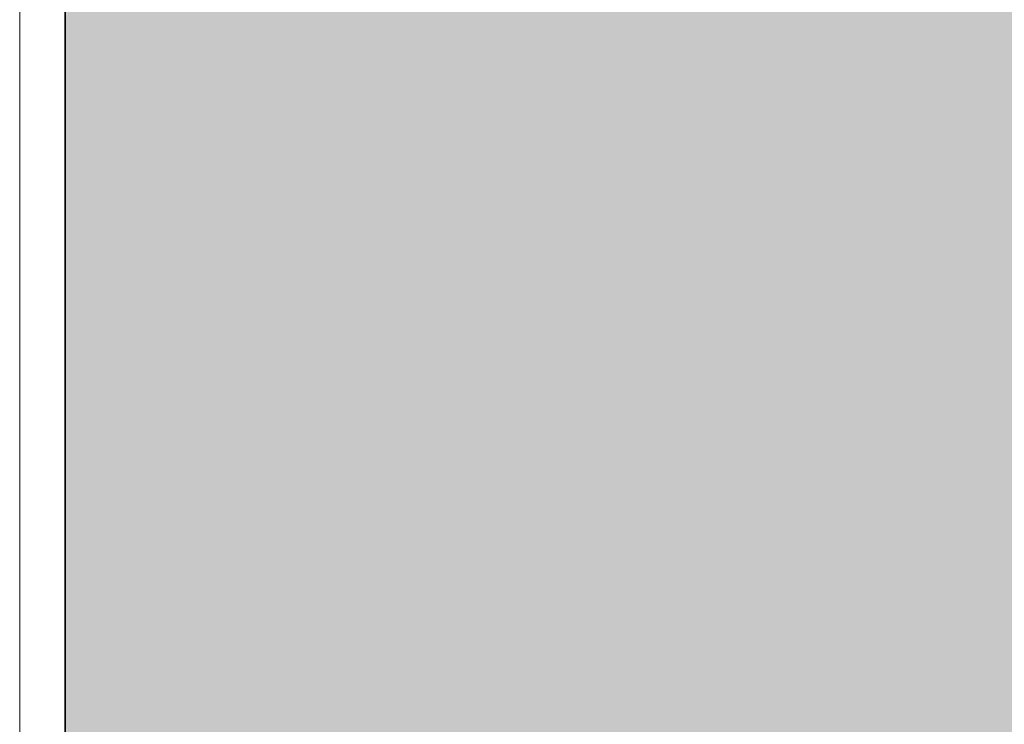
# Model space of a CAD drawing. Units: inches. Extents: x 2091 to 2899, y 967 to 2217.
# Tile 234 of 256: x 2203.1157 to 2203.7172, y 1152.6774 to 1153.1078. Entities that reach past the tile are written whole.
import ezdxf

# ---------------------------------------------------------------- set-up
doc = ezdxf.new("R2010")
doc.units = ezdxf.units.IN
doc.layers.add('A-GLAZ', color=4, linetype='Continuous', lineweight=18)
doc.layers.add('C-PROP', color=7, linetype='Continuous', lineweight=35)
doc.layers.add('A-WALL-PATT', color=141, linetype='Continuous', lineweight=13, true_color=0xadddf7)

# ---------------------------------------------------------------- blocks, each defined once
blk = doc.blocks.new('WIN-DOUBLE-LINE')
blk.add_line((0.0004, -0.00045), (0.0004, 80.8229))

msp = doc.modelspace()

# ---------------------------------------------------------------- hatches: boundary and pattern name
at = {"layer": 'A-WALL-PATT'}
h = msp.add_hatch(color=256, dxfattribs=at)
h.dxf.hatch_style = 1
h.paths.add_polyline_path([(2803.1436, 2050.91906), (2203.1436, 2050.91906), (2203.1436, 1090.91906), (2803.1436, 1090.91906)])
h.paths.add_polyline_path([(2635.79885, 1147.54046), (2674.52405, 1147.54046, 0.376086), (2678.52967, 1152.8802), (2678.52967, 1159.55647, 0.333335), (2674.52432, 1163.56185), (2674.52432, 1163.56185), (2674.52432, 1192.93439), (2635.80597, 1192.93439), (2597.08762, 1192.93439), (2597.08762, 1163.56185, 0.333335), (2593.08228, 1159.55647), (2593.08228, 1152.8802, 0.376086), (2597.08789, 1147.54046)], flags=0)
h.paths.add_polyline_path([(2436.01043, 1278.24078, 0.000483), (2435.95264, 1278.21503, -0.001328), (2435.93563, 1278.11169, -0.001711), (2436.11644, 1278.04076, 0.002185)], flags=0)
h.paths.add_polyline_path([(2794.1436, 1143.41906), (2794.1436, 1347.41906), (2543.37017, 1347.41906), (2543.37017, 1351.91906), (2794.1436, 1351.91906), (2794.1436, 1392.71355), (2793.9474, 1392.71355), (2793.9474, 1473.5369), (2794.1436, 1473.5369), (2794.1436, 1531.91906), (2650.1436, 1531.91906), (2650.1436, 1536.41906), (2794.1436, 1536.41906), (2794.1436, 1692.41906), (2609.37561, 1692.41906), (2609.37561, 1644.41906), (2604.87561, 1644.41906), (2604.87561, 1744.91906), (2609.37561, 1744.91906), (2609.37561, 1696.91906), (2794.1436, 1696.91906), (2794.1436, 1780.91906), (2609.6436, 1780.91906), (2493.87561, 1780.91906), (2493.87561, 1785.41906), (2609.6436, 1785.41906), (2794.1436, 1785.41906), (2794.1436, 1847.93882), (2793.95122, 1847.93882), (2793.95122, 1928.76217), (2794.1436, 1928.76217), (2794.1436, 1941.41906), (2614.1436, 1941.41906), (2614.1436, 1821.41906), (2609.6436, 1821.41906), (2609.6436, 1941.41906), (2392.1436, 1941.41906), (2392.1436, 1819.91906), (2387.6436, 1819.91906), (2387.6436, 1941.41906), (2212.1436, 1941.41906), (2212.1436, 1783.91906), (2392.1436, 1783.91906), (2392.1436, 1780.91906), (2212.1436, 1780.91906), (2212.1436, 1629.41906), (2387.6436, 1629.41906), (2387.6436, 1744.91906), (2392.1436, 1744.91906), (2392.1436, 1627.91906), (2317.1436, 1627.91906), (2317.1436, 1551.41906), (2317.1436, 1536.41906), (2459.38359, 1536.41906), (2459.38359, 1602.39648), (2463.88359, 1602.39648), (2463.88359, 1531.91906), (2456.6436, 1531.91906), (2456.6436, 1529.91906), (2452.1436, 1529.91906), (2452.1436, 1531.91906), (2312.6436, 1531.91906), (2312.6436, 1551.41906), (2306.1436, 1551.41906), (2306.1436, 1555.91906), (2308.1436, 1555.91906), (2308.1436, 1551.41906), (2312.6436, 1551.41906), (2312.6436, 1627.91906), (2212.1436, 1627.91906), (2212.1436, 1555.91906), (2270.1436, 1555.91906), (2270.1436, 1551.41906), (2212.1436, 1551.41906), (2212.1436, 1351.91906), (2272.1436, 1351.91906), (2272.1436, 1347.41906), (2212.1436, 1347.41906), (2212.1436, 1275.41906), (2308.1436, 1275.41906), (2308.1436, 1351.91906), (2452.1436, 1351.91906), (2452.1436, 1493.91906), (2456.6436, 1493.91906), (2456.6436, 1347.41906), (2312.6436, 1347.41906), (2312.6436, 1270.91906), (2212.1436, 1270.91906), (2212.1436, 1099.91906), (2281.23752, 1099.91906), (2282.87104, 1110.9138), (2282.00834, 1116.9966), (2278.55774, 1121.4204), (2268.20564, 1128.0562), (2272.08764, 1128.0562), (2273.81294, 1131.927), (2279.42034, 1134.6919), (2285.02784, 1135.2449), (2287.61584, 1137.4568), (2288.04714, 1138.0098), (2289.34114, 1140.7747), (2291.06654, 1139.6687), (2292.36054, 1135.2449), (2295.37984, 1136.9038), (2296.24254, 1135.7979), (2297.10524, 1133.033), (2300.12464, 1138.0098), (2303.14394, 1138.0098), (2304.43794, 1135.7979), (2303.14394, 1133.586), (2306.59464, 1134.6919), (2307.88874, 1133.033), (2310.90804, 1135.2449), (2313.92744, 1134.1389), (2315.62686, 1132.4271), (2308.32004, 1117.5496), (2290.20384, 1109.8079), (2288.90984, 1103.1721), (2289.27231, 1099.91906), (2434.91823, 1099.91906), (2431.59323, 1124.78806), (2429.93023, 1169.55306), (2430.92718, 1240.51969), (2435.65893, 1238.18613), (2437.13523, 1196.55406), (2438.79823, 1143.97306), (2442.67823, 1111.99806), (2446.55823, 1099.91906), (2794.1436, 1099.91906), (2794.1436, 1138.91906), (2548.03245, 1138.91906), (2548.03245, 1143.41906), (2548.03245, 1148.81906), (2546.66846, 1148.03156), (2528.68569, 1179.17862, 0.256256), (2512.03245, 1148.81906), (2512.03245, 1143.41906), (2512.03245, 1138.91906), (2507.53245, 1138.91906), (2507.53245, 1143.41906), (2507.53245, 1148.81906, 0.256256), (2490.8792, 1179.17862), (2472.89644, 1148.03156), (2471.53245, 1148.81906), (2471.53245, 1143.41906), (2467.03245, 1143.41906), (2467.03245, 1269.94579, 0.039061), (2460.90999, 1273.58006), (2467.03245, 1273.58006), (2467.03245, 1286.32536, 0.014511), (2465.21619, 1286.76191), (2467.03245, 1287.05258), (2467.03245, 1323.41906), (2471.53245, 1323.41906), (2471.53245, 1148.81906), (2489.53245, 1179.99597), (2490.89644, 1179.20847), (2490.8792, 1179.17862, -0.256256), (2507.53245, 1148.81906), (2507.53245, 1143.41906), (2512.03245, 1143.41906), (2512.03245, 1148.81906, -0.256256), (2528.68569, 1179.17862), (2528.66846, 1179.20847), (2530.03245, 1179.99597), (2548.03245, 1148.81906), (2548.03245, 1143.41906)], flags=16)
h.paths.add_polyline_path([(2607.76855, 1200.94508), (2607.76855, 1265.03063), (2597.08762, 1281.05201), (2619.78459, 1281.05201), (2627.79528, 1337.12686), (2635.79885, 1337.12686), (2643.81666, 1337.12686), (2651.82736, 1281.05201), (2674.52432, 1281.05201), (2663.8434, 1265.03063), (2663.8434, 1200.94508), (2635.80597, 1200.94508)], flags=0)
edge = h.paths.add_edge_path(flags=0)
edge.add_ellipse((13303.89622, 1272.99872), major_axis=(-10595.31304, 0), ratio=0.84230387009, start_angle=0.628237219, end_angle=0.6465541, ccw=False)
edge.add_ellipse((2711.70045, 1156.85268), major_axis=(2.21977, 0), ratio=0.8423039, start_angle=111.53524, end_angle=180.62824, ccw=False)
edge.add_ellipse((13303.15629, 1272.99872), major_axis=(-10593.02631, 0), ratio=0.84230386954, start_angle=0.528271472, end_angle=0.646554097, ccw=False)
edge.add_line((2710.7646, 1175.3333), (2710.12999, 1175.3333))
edge.add_ellipse((2710.12999, 1176.57978), major_axis=(1.47985, 0), ratio=0.8423039, start_angle=180, end_angle=270, ccw=False)
edge.add_line((2708.65014, 1176.57978), (2708.65014, 1200.78291))
edge.add_ellipse((2710.12999, 1200.78291), major_axis=(1.47985, 0), ratio=0.8423039, start_angle=90, end_angle=180, ccw=False)
edge.add_line((2710.12999, 1202.02939), (2710.46508, 1202.02939))
edge.add_ellipse((13303.15629, 1272.99872), major_axis=(-10593.02631, 0), ratio=0.84230386954, start_angle=-0.090229089, end_angle=0.383866779, ccw=False)
edge.add_ellipse((2710.12999, 1290.92703), major_axis=(-1.47985, 0), ratio=0.8423039, start_angle=0, end_angle=90, ccw=False)
edge.add_line((2708.65014, 1290.92703), (2708.65014, 1315.13017))
edge.add_ellipse((2710.12999, 1315.13017), major_axis=(-1.47985, 0), ratio=0.8423039, start_angle=-90, end_angle=0, ccw=False)
edge.add_line((2710.12999, 1316.37665), (2710.70631, 1316.37665))
edge.add_ellipse((3238.40172, 1296.28957), major_axis=(528.234, 0), ratio=0.84230387, start_angle=176.3495724, end_angle=177.8200497, ccw=False)
edge.add_ellipse((2775.06304, 1071.4507), major_axis=(313.30776, 0), ratio=0.84230387, start_angle=102.1259656, end_angle=103.780529, ccw=False)
edge.add_ellipse((2775.06304, 1078.3057), major_axis=(-305.30289, 0), ratio=0.84230387, start_angle=-79.790461, end_angle=-77.5553727, ccw=False)
edge.add_ellipse((2695.14177, 1541.97538), major_axis=(-250.96022, 0), ratio=0.84230387, start_angle=99.256566, end_angle=102.5549326)
edge.add_line((2741.41033, 1334.21426), (2747.13255, 1337.37848))
edge.add_ellipse((2747.53862, 1336.85748), major_axis=(-0.73992, 0), ratio=0.842304, start_angle=270, end_angle=307.93313, ccw=False)
edge.add_ellipse((2747.53862, 1336.85748), major_axis=(-0.73992, 0), ratio=0.842304, start_angle=232.06687, end_angle=270, ccw=False)
edge.add_line((2747.94469, 1337.37848), (2753.66691, 1334.21426))
edge.add_ellipse((2799.93547, 1541.97538), major_axis=(250.96022, 0), ratio=0.84230387, start_angle=257.4450674, end_angle=260.743434)
edge.add_ellipse((2720.01419, 1078.3057), major_axis=(305.30289, 0), ratio=0.84230387, start_angle=77.5553727, end_angle=79.790461, ccw=False)
edge.add_ellipse((2720.01419, 1071.4507), major_axis=(-313.30776, 0), ratio=0.84230387, start_angle=256.219471, end_angle=257.8740344, ccw=False)
edge.add_ellipse((2256.67551, 1296.28957), major_axis=(-528.234, 0), ratio=0.84230387, start_angle=182.1799503, end_angle=183.6504276, ccw=False)
edge.add_line((2784.37092, 1316.37665), (2784.94725, 1316.37665))
edge.add_ellipse((2784.94725, 1315.13017), major_axis=(1.47985, 0), ratio=0.8423039, start_angle=0, end_angle=90, ccw=False)
edge.add_line((2786.42709, 1315.13017), (2786.42709, 1290.92703))
edge.add_ellipse((2784.94725, 1290.92703), major_axis=(1.47985, 0), ratio=0.8423039, start_angle=270, end_angle=360, ccw=False)
edge.add_ellipse((-7808.07906, 1272.99872), major_axis=(10593.02631, 0), ratio=0.84230386954, start_angle=-0.383866779, end_angle=0.090229089, ccw=False)
edge.add_line((2784.61216, 1202.02939), (2784.94725, 1202.02939))
edge.add_ellipse((2784.94725, 1200.78291), major_axis=(1.47985, 0), ratio=0.8423039, start_angle=0, end_angle=90, ccw=False)
edge.add_line((2786.42709, 1200.78291), (2786.42709, 1176.57978))
edge.add_ellipse((2784.94725, 1176.57978), major_axis=(-1.47985, 0), ratio=0.8423039, start_angle=90, end_angle=180, ccw=False)
edge.add_line((2784.94725, 1175.3333), (2784.31264, 1175.3333))
edge.add_ellipse((-7808.07906, 1272.99872), major_axis=(10593.02631, 0), ratio=0.84230386954, start_angle=-0.618643196, end_angle=-0.528271472, ccw=False)
edge.add_ellipse((2783.37678, 1156.85268), major_axis=(-2.21977, 0), ratio=0.8423039, start_angle=179.37176, end_angle=248.46476, ccw=False)
edge.add_ellipse((-7808.81898, 1272.99872), major_axis=(-10595.31304, 0), ratio=0.84230386576, start_angle=179.353445923, end_angle=179.371762803, ccw=False)
edge.add_ellipse((2780.2973, 1153.50079), major_axis=(-5.24643, 0), ratio=0.8423039, start_angle=90, end_angle=179.35345, ccw=False)
edge.add_line((2780.2973, 1149.08171), (2714.77993, 1149.08171))
edge.add_ellipse((2714.77993, 1153.50079), major_axis=(5.24643, 0), ratio=0.8423039, start_angle=180.64655, end_angle=270, ccw=False)
edge = h.paths.add_edge_path(flags=0)
edge.add_line((2718.18737, 1151.00783), (2718.18737, 1170.47236))
edge.add_ellipse((2721.14706, 1170.47236), major_axis=(-2.95969, 0), ratio=0.8423039, start_angle=-90, end_angle=0, ccw=False)
edge.add_line((2721.14706, 1172.96532), (2773.93017, 1172.96532))
edge.add_ellipse((2773.93017, 1170.47236), major_axis=(-2.95969, 0), ratio=0.8423039, start_angle=180, end_angle=270, ccw=False)
edge.add_line((2776.88987, 1170.47236), (2776.88987, 1151.00783))
edge.add_line((2776.88987, 1151.00783), (2718.18737, 1151.00783))
edge = h.paths.add_edge_path(flags=0)
edge.add_line((2718.18737, 1180.23415), (2718.18737, 1199.05783))
edge.add_ellipse((2747.53862, 1320.39864), major_axis=(147.01792, 0), ratio=0.84230387, start_angle=256.4018653, end_angle=283.5981347)
edge.add_line((2776.88987, 1199.05783), (2776.88987, 1180.23415))
edge.add_ellipse((2747.53862, 1301.57496), major_axis=(147.01792, 0), ratio=0.84230387, start_angle=256.4018653, end_angle=283.5981347, ccw=False)
edge = h.paths.add_edge_path(flags=0)
edge.add_ellipse((13303.15629, 1272.99872), major_axis=(-10591.54646, 0), ratio=0.84230386955, start_angle=0.055594314, end_angle=0.377764194, ccw=False)
edge.add_line((2711.61686, 1262.72171), (2715.66741, 1249.4954))
edge.add_ellipse((6413.89196, 1241.69192), major_axis=(-3698.23616, 0), ratio=0.8423038695, start_angle=-0.12089737, end_angle=0.36407635)
edge.add_line((2715.76104, 1218.19245), (2711.93431, 1203.16736))
edge = h.paths.add_edge_path(flags=0)
edge.add_line((2718.18737, 1251.07457), (2716.00249, 1267.45044))
edge.add_ellipse((2742.15117, 1202.18954), major_axis=(81.77258, 0), ratio=0.84230387, start_angle=94.277421, end_angle=111.8349538, ccw=False)
edge.add_line((2737.00975, 1270.93063), (2758.06748, 1270.93063))
edge.add_ellipse((2752.92606, 1202.18954), major_axis=(81.77258, 0), ratio=0.84230387, start_angle=68.1650462, end_angle=85.722579, ccw=False)
edge.add_line((2779.07475, 1267.45044), (2776.88987, 1251.07457))
edge.add_ellipse((2750.33806, 1187.88536), major_axis=(79.57966, 0), ratio=0.84230387, start_angle=67.2080851, end_angle=85.1299304)
edge.add_line((2756.03466, 1254.74366), (2739.04258, 1254.74366))
edge.add_ellipse((2744.73917, 1187.88536), major_axis=(79.57966, 0), ratio=0.84230387, start_angle=94.8700696, end_angle=112.7919149)
edge = h.paths.add_edge_path(flags=0)
edge.add_line((2783.14293, 1203.16736), (2779.31619, 1218.19245))
edge.add_ellipse((-918.81473, 1241.69192), major_axis=(3698.23616, 0), ratio=0.8423038695, start_angle=-0.36407635, end_angle=0.12089737)
edge.add_line((2779.40983, 1249.4954), (2783.46037, 1262.72171))
edge.add_ellipse((-7808.07906, 1272.99872), major_axis=(-10591.54646, 0), ratio=0.84230386954, start_angle=179.622235806, end_angle=179.944405687, ccw=False)
edge = h.paths.add_edge_path(flags=0)
edge.add_ellipse((2734.20089, 1286.69044), major_axis=(-0.35661, 6.34008), ratio=0.6038336, start_angle=89.002014, end_angle=253.657408, ccw=False)
edge.add_line((2730.369, 1286.54181), (2730.369, 1301.35198))
edge.add_line((2730.369, 1301.35198), (2735.91331, 1305.2148))
edge.add_ellipse((2736.38492, 1304.73456), major_axis=(0.73992, 0), ratio=0.842304, start_angle=90, end_angle=134.48021, ccw=False)
edge.add_line((2736.38492, 1305.3578), (2738.03278, 1305.3578))
edge.add_line((2738.03278, 1305.3578), (2738.03278, 1307.70793))
edge.add_ellipse((2794.20164, 1307.70793), major_axis=(56.16886, 0), ratio=0.84230387, start_angle=150.56143, end_angle=180, ccw=False)
edge.add_ellipse((2700.87559, 1307.70793), major_axis=(-56.16886, 0), ratio=0.84230387, start_angle=180, end_angle=209.43857, ccw=False)
edge.add_line((2757.04445, 1307.70793), (2757.04445, 1305.3578))
edge.add_line((2757.04445, 1305.3578), (2758.69232, 1305.3578))
edge.add_ellipse((2758.69232, 1304.73456), major_axis=(-0.73992, 0), ratio=0.842304, start_angle=225.51979, end_angle=270, ccw=False)
edge.add_line((2759.16392, 1305.2148), (2764.70823, 1301.35198))
edge.add_line((2764.70823, 1301.35198), (2764.70823, 1286.54181))
edge.add_ellipse((2760.87634, 1286.69044), major_axis=(0.35661, 6.34008), ratio=0.6038336, start_angle=106.342592, end_angle=270.997986, ccw=False)
edge.add_line((2757.04445, 1285.79709), (2757.04445, 1307.70793))
edge.add_ellipse((2700.87559, 1307.70793), major_axis=(-56.16886, 0), ratio=0.84230387, start_angle=180, end_angle=209.43857)
edge.add_ellipse((2794.20164, 1307.70793), major_axis=(56.16886, 0), ratio=0.84230387, start_angle=150.56143, end_angle=180)
edge.add_line((2738.03278, 1307.70793), (2738.03278, 1285.79709))
h.paths.add_polyline_path([(2417.81227, 1104.4497), (2413.49227, 1102.5297), (2410.61227, 1103.9697), (2409.17227, 1106.3697), (2407.25227, 1107.3297), (2406.29227, 1109.7297), (2405.33227, 1114.0497), (2405.33227, 1117.8897), (2406.29227, 1120.1297), (2407.25227, 1119.8097), (2408.84832, 1118.32766), (2410.17395, 1119.42417), (2410.21127, 1120.4057), (2411.04073, 1121.41905), (2410.69927, 1119.8587), (2410.17395, 1119.42417), (2410.08845, 1117.17611), (2411.13284, 1116.20632), (2413.97227, 1119.3297), (2416.85227, 1120.7697), (2416.86972, 1120.79878), (2417.03507, 1119.40512), (2417.89621, 1118.14338), (2418.29227, 1118.3697), (2419.54445, 1120.03927), (2419.36092, 1118.38749), (2419.03211, 1119.35615), (2418.39894, 1118.51193), (2419.25227, 1114.5297), (2418.79409, 1107.19879)], flags=0)
h.paths.add_polyline_path([(2508.87017, 1347.41906), (2508.37017, 1347.41906), (2508.37017, 1351.91906), (2508.87017, 1351.91906)], flags=0)
h.paths.add_polyline_path([(2473.37017, 1347.41906), (2472.37017, 1347.41906), (2467.87017, 1347.41906), (2467.87017, 1455.41906), (2472.37017, 1455.41906), (2472.37017, 1352.41906), (2473.37017, 1352.41906)], flags=0)
h.paths.add_polyline_path([(2352.10624, 1217.4462), (2349.22624, 1218.8862), (2347.78624, 1221.2862), (2345.86624, 1222.2462), (2344.90624, 1224.6462), (2343.94624, 1228.9662), (2343.94624, 1232.8062), (2344.90624, 1235.0462), (2345.86624, 1234.7262), (2347.46229, 1233.24415), (2348.78792, 1234.34066), (2348.82524, 1235.3222), (2349.6547, 1236.33555), (2349.31324, 1234.7752), (2348.78792, 1234.34066), (2348.70242, 1232.0926), (2349.74681, 1231.12282), (2352.58624, 1234.2462), (2355.46624, 1235.6862), (2355.48369, 1235.71528), (2355.64904, 1234.32161), (2356.51018, 1233.05988), (2356.90624, 1233.2862), (2358.15842, 1234.95576), (2357.97489, 1233.30398), (2357.64608, 1234.27264), (2357.01291, 1233.42842), (2357.86624, 1229.4462), (2357.40806, 1222.11529), (2356.42624, 1219.3662)], flags=0)
h.paths.add_polyline_path([(2348.2968, 1112.22442), (2347.0138, 1112.31042), (2345.5298, 1114.12742), (2345.7318, 1115.85842), (2346.8118, 1116.98242), (2346.8118, 1114.64642), (2345.8668, 1114.21442), (2346.8798, 1114.30042)], flags=0)
h.paths.add_polyline_path([(2347.0138, 1110.92642), (2346.2718, 1110.49342), (2346.6098, 1111.18642)], flags=0)
h.paths.add_polyline_path([(2345.8668, 1118.19442), (2345.5298, 1117.32942), (2343.7078, 1118.02142), (2344.3828, 1118.62642)], flags=0)
h.paths.add_polyline_path([(2346.6768, 1109.28242), (2346.0698, 1108.07142), (2345.8668, 1110.06142)], flags=0)
h.paths.add_polyline_path([(2345.0568, 1119.75142), (2343.6398, 1119.75142), (2343.9778, 1121.13542)], flags=0)
h.paths.add_polyline_path([(2345.2598, 1116.55042), (2345.1248, 1115.85842), (2344.9218, 1115.68542), (2344.7198, 1116.37742)], flags=0)
h.paths.add_polyline_path([(2345.6648, 1112.31042), (2345.4618, 1111.53242), (2344.0448, 1111.96442), (2344.6518, 1112.57042)], flags=0)
h.paths.add_polyline_path([(2345.1918, 1113.34942), (2344.4498, 1113.86842), (2344.7198, 1114.38742)], flags=0)
h.paths.add_polyline_path([(2344.6518, 1116.80942), (2344.1798, 1115.68542), (2344.6518, 1115.33942), (2343.9098, 1114.90642), (2343.0328, 1115.94442), (2343.6398, 1116.46342)], flags=0)
h.paths.add_polyline_path([(2345.8668, 1106.68642), (2344.9898, 1105.56242), (2344.5168, 1106.60042)], flags=0)
h.paths.add_polyline_path([(2344.8548, 1110.06142), (2344.5168, 1109.28242), (2344.1128, 1109.71542)], flags=0)
h.paths.add_polyline_path([(2344.0448, 1113.52242), (2343.4378, 1113.08942), (2342.7628, 1113.95442)], flags=0)
h.paths.add_polyline_path([(2344.3148, 1111.01242), (2342.9648, 1110.32042), (2342.9648, 1111.09942)], flags=0)
h.paths.add_polyline_path([(2345.1248, 1104.69742), (2344.5848, 1103.74542), (2344.4498, 1104.26442)], flags=0)
h.paths.add_polyline_path([(2342.8298, 1121.22242), (2341.7498, 1120.53042), (2340.5358, 1121.04942), (2340.1308, 1121.82842), (2340.6708, 1122.95242), (2341.1428, 1121.82842), (2341.6148, 1122.00142)], flags=0)
h.paths.add_polyline_path([(2342.9648, 1119.75142), (2343.0328, 1118.45342), (2342.0878, 1118.02142), (2342.0198, 1119.49142)], flags=0)
h.paths.add_polyline_path([(2342.6948, 1116.89642), (2341.9528, 1116.63642), (2342.0198, 1117.32942)], flags=0)
h.paths.add_polyline_path([(2343.0328, 1112.22442), (2342.0198, 1111.79142), (2341.5478, 1112.22442), (2342.3578, 1113.34942)], flags=0)
h.paths.add_polyline_path([(2343.7748, 1104.43742), (2342.6278, 1102.88042), (2342.6948, 1104.61042), (2343.4378, 1105.12942)], flags=0)
h.paths.add_polyline_path([(2342.0198, 1115.07942), (2340.8058, 1115.51242), (2340.9408, 1116.37742)], flags=0)
h.paths.add_polyline_path([(2341.4808, 1120.09742), (2341.4808, 1119.40542), (2341.0758, 1119.57842), (2341.1428, 1120.09742)], flags=0)
h.paths.add_polyline_path([(2341.8178, 1114.47342), (2340.9408, 1113.08942), (2340.8058, 1114.56042)], flags=0)
h.paths.add_polyline_path([(2341.1428, 1118.54042), (2340.9408, 1116.98242), (2339.0508, 1117.67542), (2339.0508, 1118.62642)], flags=0)
h.paths.add_polyline_path([(2342.6948, 1101.66842), (2341.9528, 1101.84142), (2342.5598, 1102.36142)], flags=0)
h.paths.add_polyline_path([(2340.3328, 1119.66542), (2338.4438, 1119.57842), (2337.9038, 1120.35742), (2339.6578, 1120.61642)], flags=0)
h.paths.add_polyline_path([(2340.3328, 1115.33942), (2340.0628, 1113.69542), (2339.3878, 1115.33942)], flags=0)
h.paths.add_polyline_path([(2341.8178, 1103.83142), (2341.5478, 1102.88042), (2341.1428, 1103.65842)], flags=0)
h.paths.add_polyline_path([(2339.0508, 1122.86642), (2337.2958, 1121.82842), (2337.0938, 1123.12542), (2337.7688, 1123.81842)], flags=0)
h.paths.add_polyline_path([(2339.1178, 1121.74142), (2338.8478, 1121.22242), (2338.1738, 1121.04942), (2338.3758, 1121.56842)], flags=0)
h.paths.add_polyline_path([(2339.1858, 1119.31942), (2338.6458, 1118.71342), (2338.2408, 1118.10742), (2338.2408, 1118.88642)], flags=0)
h.paths.add_polyline_path([(2341.1428, 1101.92842), (2340.6028, 1101.23642), (2340.0628, 1101.84142), (2340.6028, 1102.36142)], flags=0)
h.paths.add_polyline_path([(2337.6338, 1117.76142), (2336.6208, 1118.28042), (2337.2958, 1118.97242)], flags=0)
h.paths.add_polyline_path([(2336.8238, 1119.57842), (2334.7988, 1118.97242), (2335.2038, 1120.35742), (2336.5538, 1120.87642)], flags=0)
h.paths.add_polyline_path([(2339.1178, 1100.45742), (2337.3638, 1100.54342), (2336.7558, 1101.23642)], flags=0)
h.paths.add_polyline_path([(2336.3508, 1122.43342), (2336.0138, 1121.91442), (2334.9338, 1122.43342), (2334.5288, 1123.47142), (2335.7438, 1122.77942)], flags=0)
h.paths.add_polyline_path([(2334.7318, 1120.87642), (2334.2588, 1120.35742), (2334.0568, 1120.78942), (2334.5968, 1121.30842)], flags=0)
h.paths.add_polyline_path([(2334.4618, 1122.17442), (2332.5718, 1121.30842), (2331.3568, 1122.17442), (2332.0998, 1122.86642)], flags=0)
h.paths.add_polyline_path([(2334.2588, 1118.54042), (2333.3818, 1118.45342), (2333.6518, 1119.31942)], flags=0)
h.paths.add_polyline_path([(2335.5418, 1102.27442), (2334.1918, 1102.62042), (2335.2718, 1103.31242)], flags=0)
h.paths.add_polyline_path([(2332.7068, 1119.66542), (2331.6948, 1120.44342), (2332.5048, 1120.78942)], flags=0)
h.paths.add_polyline_path([(2334.7318, 1101.14942), (2333.5168, 1101.58242), (2333.9888, 1101.75542)], flags=0)
h.paths.add_polyline_path([(2332.6398, 1116.63642), (2331.0868, 1116.29042), (2331.9648, 1118.19442)], flags=0)
h.paths.add_polyline_path([(2330.7498, 1121.56842), (2330.2768, 1120.27042), (2328.5228, 1119.31942), (2328.9948, 1121.04942)], flags=0)
h.paths.add_polyline_path([(2330.7498, 1118.62642), (2330.0078, 1117.50242), (2329.8728, 1118.02142)], flags=0)
h.paths.add_polyline_path([(2332.0998, 1102.36142), (2330.5468, 1102.01442), (2331.6948, 1102.96642)], flags=0)
h.paths.add_polyline_path([(2329.5348, 1113.60842), (2329.0628, 1112.31042), (2328.5898, 1113.34942)], flags=0)
h.paths.add_polyline_path([(2328.3878, 1117.84842), (2327.5098, 1116.55042), (2327.1728, 1117.76142)], flags=0)
h.paths.add_polyline_path([(2329.7378, 1106.51342), (2329.5348, 1105.30242), (2328.2528, 1106.08142)], flags=0)
h.paths.add_polyline_path([(2328.6578, 1114.38742), (2328.0498, 1114.12742), (2328.3198, 1114.90642)], flags=0)
h.paths.add_polyline_path([(2328.3198, 1112.22442), (2327.1058, 1112.13742), (2326.7008, 1112.65642)], flags=0)
h.paths.add_polyline_path([(2326.9028, 1115.25242), (2326.7008, 1114.12742), (2325.2158, 1113.60842), (2326.0928, 1115.33942)], flags=0)
h.paths.add_polyline_path([(2326.6328, 1108.33042), (2326.0928, 1107.37942), (2325.8908, 1108.50342), (2326.4978, 1109.10942)], flags=0)
h.paths.add_polyline_path([(2615.1436, 1531.91906), (2609.6436, 1531.91906), (2609.6436, 1620.41906), (2614.1436, 1620.41906), (2614.1436, 1536.41906), (2615.1436, 1536.41906)], flags=0)
h.paths.add_polyline_path([(2545.1436, 1563.41906), (2464.1436, 1563.41906), (2464.1436, 1632.41906), (2509.1436, 1632.41906), (2509.1436, 1627.91906), (2509.1436, 1603.91906), (2468.6436, 1603.91906), (2468.6436, 1567.91906), (2540.6436, 1567.91906), (2540.6436, 1591.91906), (2545.1436, 1591.91906)], flags=0)
h.paths.add_polyline_path([(2388.96905, 1549.98573), (2357.43418, 1549.98573), (2357.43418, 1623.36078), (2399.36278, 1623.36078), (2435.68947, 1623.36078), (2435.59255, 1602.55927), (2435.59255, 1602.39648), (2388.96905, 1602.39648)], flags=0)
h.paths.add_polyline_path([(2388.88063, 1555.80915), (2374.90443, 1555.80915), (2374.90443, 1600.57156), (2374.90443, 1615.45765), (2406.35088, 1615.45765), (2406.35088, 1618.93943), (2412.17429, 1615.45765), (2406.35088, 1611.97586), (2406.35088, 1615.45765), (2388.88063, 1615.45765)], flags=0)
h.paths.add_polyline_path([(2568.87561, 1644.41906), (2453.37561, 1644.41906), (2453.37561, 1785.41906), (2457.87561, 1785.41906), (2457.87561, 1648.91906), (2568.87561, 1648.91906)], flags=0)
h.paths.add_polyline_path([(2212.1436, 1945.91906), (2212.1436, 2041.91906), (2794.1436, 2041.91906), (2794.1436, 1945.91906)], flags=16)
h.paths.add_polyline_path([(2271.08273, 1964.31724), (2776.85297, 1964.31724), (2776.85297, 2037.16962), (2271.08273, 2037.16962)], flags=8)
h.paths.add_polyline_path([(2380.64929, 1536.82414), (2461.04081, 1536.82414), (2461.04081, 1554.65259), (2380.64929, 1554.65259)], flags=8)
h.paths.add_polyline_path([(2240.75571, 1609.72545), (2309.18583, 1609.72545), (2309.18583, 1617.6982), (2240.75571, 1617.6982)], flags=8)
h.paths.add_polyline_path([(2212.67726, 1313.5041), (2282.59152, 1313.5041), (2282.59152, 1322.74524), (2212.67726, 1322.74524)], flags=8)
h.paths.add_polyline_path([(2457.11198, 1114.77857), (2558.48158, 1114.77857), (2558.48158, 1142.21968), (2457.11198, 1142.21968)], flags=8)
h.paths.add_polyline_path([(2473.44234, 1273.01007), (2604.64123, 1273.01007), (2604.64123, 1318.34693), (2473.44234, 1318.34693)], flags=8)
h.paths.add_polyline_path([(2638.8763, 1626.97743), (2684.25037, 1627.97674), (2684.03848, 1637.59749), (2638.66442, 1636.59819)], flags=8)
h.paths.add_polyline_path([(2537.59055, 1453.79345), (2628.38955, 1453.79345), (2628.38955, 1475.34481), (2537.59055, 1475.34481)], flags=8)
h.paths.add_polyline_path([(2504.13764, 1714.6324), (2554.64719, 1714.6324), (2554.64719, 1730.23771), (2504.13764, 1730.23771)], flags=8)
h.paths.add_polyline_path([(2487.50118, 1575.65187), (2535.09712, 1575.65187), (2535.09712, 1598.37765), (2487.50118, 1598.37765)], flags=8)
h.paths.add_polyline_path([(2709.0994, 1735.71028), (2740.0166, 1735.71028), (2740.0166, 1749.93764), (2709.0994, 1749.93764)], flags=8)
h.paths.add_polyline_path([(2442.43842, 1792.17166), (2564.72884, 1792.17166), (2564.72884, 1842.00016), (2442.43842, 1842.00016)], flags=8)
h.paths.add_polyline_path([(2655.8158, 1809.64408), (2789.52014, 1806.6938), (2790.08498, 1832.29164), (2656.38064, 1835.24192)], flags=8)
h.paths.add_polyline_path([(2234.8427, 1797.72014), (2368.59285, 1794.76885), (2369.16072, 1820.50413), (2235.41056, 1823.45542)], flags=8)
h.paths.add_polyline_path([(2245.13847, 1644.00633), (2398.42773, 1640.6239), (2398.99484, 1666.32482), (2245.70557, 1669.70725)], flags=8)
h.paths.add_polyline_path([(2306.14285, 1431.16852), (2413.76831, 1428.79369), (2414.33315, 1454.39153), (2306.70768, 1456.76636)], flags=8)
h.paths.add_polyline_path([(2306.83458, 1458.23314), (2393.38048, 1456.32345), (2393.93281, 1481.35436), (2307.38691, 1483.26405)], flags=8)

# ---------------------------------------------------------------- linework, layer by layer
at = {"layer": 'C-PROP'}
msp.add_lwpolyline([(2203.1436, 2050.91906), (2803.1436, 2050.91906), (2803.1436, 1090.91906), (2203.1436, 1090.91906)], close=True, dxfattribs=at)

# ---------------------------------------------------------------- block references
at = {"layer": 'A-GLAZ'}
msp.add_blockref('WIN-DOUBLE-LINE', (2203.11534, 1152.2475), dxfattribs=at)

doc.saveas('drawing.dxf')
